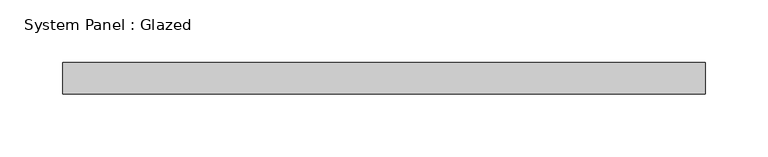
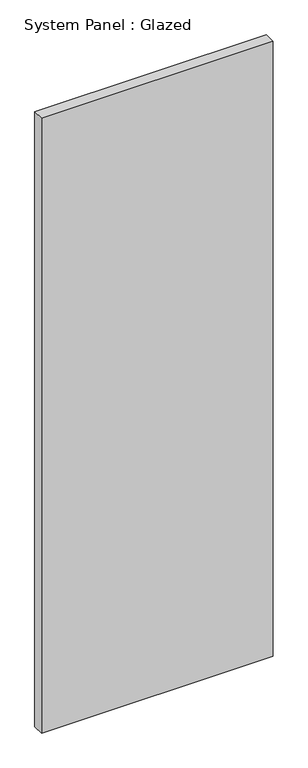
"""IFC4 building model written with IfcOpenShell, lengths in millimetres: plate geometry, System Panel : Glazed."""

from ifc_helpers import new_model, si_unit, origin, origin_with_axes, place, context, project, spatial, polyline, outline, extrude, source, transform, mapped, element, save


def system_panel_glazed_79a5eb44(model_context):
    return source(origin(), model_context, "Body", "SweptSolid", [
        extrude(outline(polyline([(257.175, 19.05), (-257.175, 19.05), (-257.175, 44.45), (257.175, 44.45), (257.175, 19.05)])), origin_with_axes(), (0.0, 0.0, 1.0), 1442.7635787),
    ])


if __name__ == "__main__":
    model = new_model("IFC4")
    model_context = context("Model", 3, world=origin())
    ifc_project = project(units=[si_unit("LENGTHUNIT", "METRE", prefix="MILLI")], contexts=[model_context])
    site = spatial("IfcSite", under=ifc_project)
    building = spatial("IfcBuilding", under=site)
    placement = place(None, origin())
    system_panel_glazed_shape = system_panel_glazed_79a5eb44(model_context)
    element("IfcPlate", 1, ObjectType="System Panel : Glazed", at=placement, inside=building, context=model_context, shape_type="MappedRepresentation", body=[
        mapped(system_panel_glazed_shape, transform((0.0, 0.0, 0.0), x_axis=(1.0, 0.0, 0.0), y_axis=(0.0, 1.0, 0.0), z_axis=(0.0, 0.0, 1.0))),
    ])
    save(model, "model.ifc")

# Revit data of these elements
# Type "System Panel : Glazed"
#   Construction Type Id = "GSP4R"
#   Analytic Construction = "1/8 in Pilkington single glazing"
#   Visual Light Transmittance = 0.9
#   Solar Heat Gain Coefficient = 0.86
#   Heat Transfer Coefficient (U) = 1.18115 BTU/(h·ft²·°F)
#   Define Thermal Properties by = 1
# Element 1 (IfcPlate, "System Panel : Glazed")
#   Materials on its faces: "Glass"
# Materials
#   "Glass": class "Glass", colour RGB 0 128 192, transparency 0.75, Description = "Soda Lime Glass", Cost = 0
